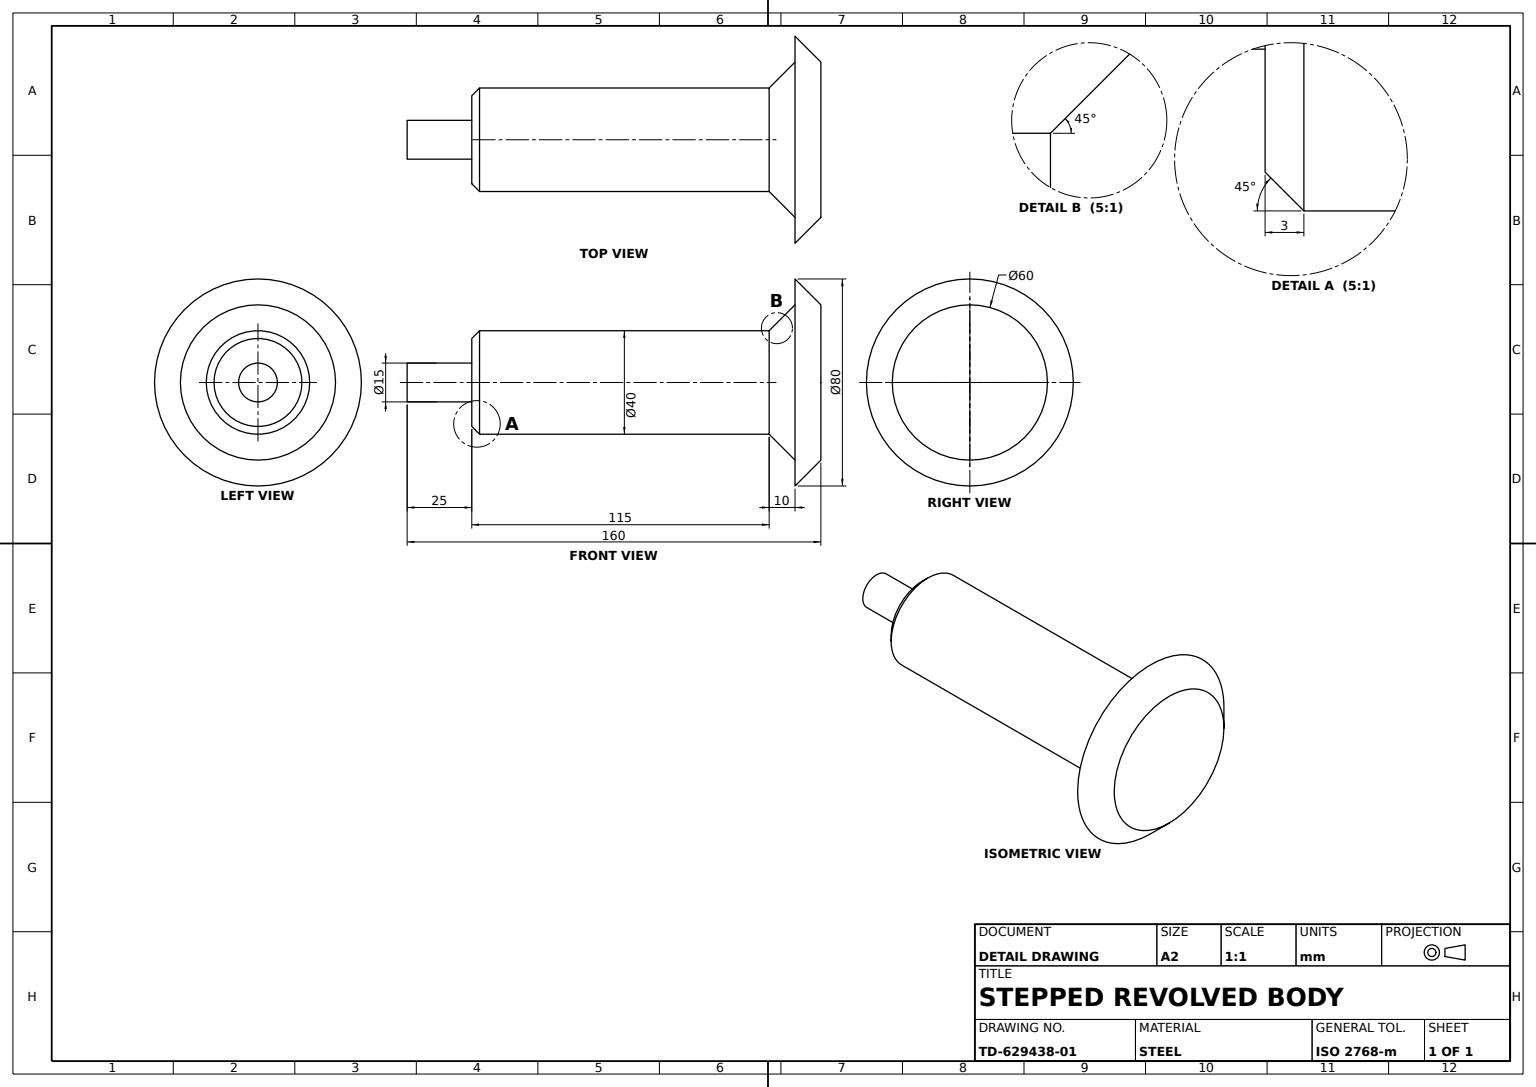
SolidWorks part; units mm, degrees
material "Plain Carbon Steel"
ref_plane "Front Plane" through (0, 0, 0) normal (0, 0, 1) x (1, 0, 0)
ref_plane "Top Plane" through (0, 0, 0) normal (0, 1, 0) x (1, 0, 0)
ref_plane "Right Plane" through (0, 0, 0) normal (1, 0, 0) x (0, 0, -1)
sketch "Plunger Profile Sketch" plane through (0, 0, 0) normal (0, 0, 1) x (1, 0, 0)
  line L0 (-51.8095, 0) -> (68.7008, 0) construction
  line L1 (0, 33.425) -> (0, -30.9725) construction
  line L2 (-35.8318, 0) -> (-35.8318, 7.5)
  line L3 (-35.8318, 7.5) -> (-10.8318, 7.5)
  line L4 (-10.8318, 7.5) -> (-10.8318, 20)
  line L5 (-7.8318, 20) -> (104.1682, 20)
  line L6 (104.1682, 20) -> (114.1682, 30)
  line L7 (114.1682, 30) -> (114.1682, 40)
  line L8 (114.1682, 40) -> (124.1682, 30)
  line L9 (124.1682, 30) -> (124.1682, 0)
  line L10 (114.1682, 30) -> (114.1682, 0)
  line L11 (104.1682, 20) -> (104.1682, 0)
  line L12 (-10.8318, 7.5) -> (-10.8318, 0)
  line L13 (68.7008, 0) -> (149.7751, 0) construction
  line L14 (124.1682, 30) -> (124.1682, 51.5671) construction
  line L15 (-35.8318, 0) -> (124.1682, 0)
  line L16 (-7.8318, 20) -> (-7.8318, 0)
  line L17 (-7.8318, 20) -> (-10.8318, 17)
  dimension "D1" = 7.5
  dimension "D2" = 25
  dimension "D3" = 20
  dimension "D4" = 115
  dimension "D5" = 10
  dimension "D6" = 10
  dimension "D7" = 40
  dimension "D8" = 45
  dimension "D9" = 3
  dimension "D10" = 45
  dimension "D11" = 35.8318
  dimension "D12" = 20
  dimension "D13" = 21.5671
  dimension "D14" = 51.8095
  dimension "D15" = 68.7008
revolve "Plunger Body Revolve" add sketch "Plunger Profile Sketch" angle 360 about L0
